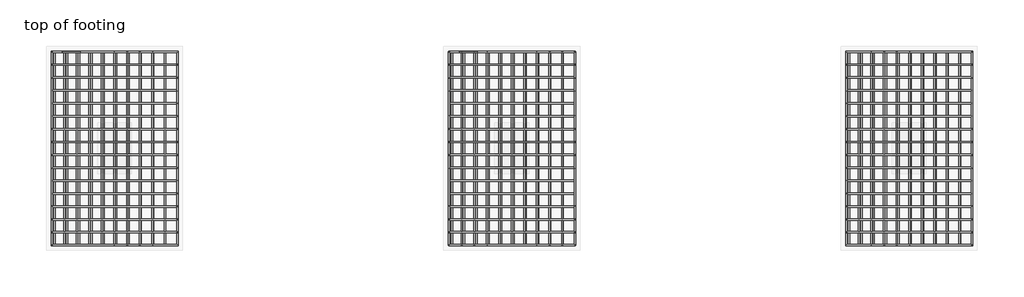
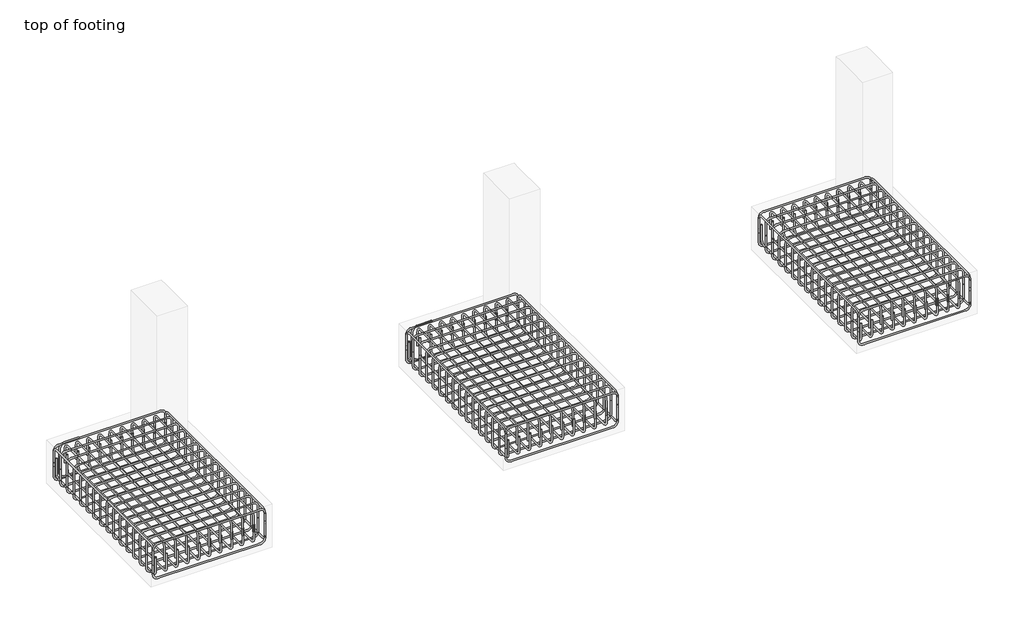
# One storey, part 2 of 8: 14 reinforcing bars.
"""IFC4 building model written with IfcOpenShell, lengths in millimetres."""

from ifc_helpers import new_model, si_unit, point, frame, origin, place, context, project, spatial, polyline, circle_curve, trimmed, segment, composite_curve, source, transform, mapped, element, save
from ifc_brep_helpers import swept_disk

model = new_model("IFC4")

# Units and contexts
model_context = context("Model", 3, world=origin())
ifc_project = project(units=[si_unit("LENGTHUNIT", "METRE", prefix="MILLI")], contexts=[model_context])

# Site, building, storey
site = spatial("IfcSite", under=ifc_project)
building = spatial("IfcBuilding", under=site)
storey = spatial("IfcBuildingStorey", under=building, Name="top of footing", Elevation=-1828.8)

# Reinforcing bars
placement = place(None, origin())
reinforcing_bar_shape = source(origin(), model_context, "Body", "SolidModel", [
    swept_disk(composite_curve([segment(polyline([(-10685.4300189, 4682.8075251, -2014.4920065), (-10685.4300189, 4682.8075251, -2161.7920065)]), True, "CONTINUOUS"), segment(trimmed(circle_curve(frame((-10685.4300189, 4729.1575251, -2161.7920065), z_axis=(1.0, 0.0, 0.0), x_axis=(0.0, -46.350000000000364, 0.0)), 46.35), [point((-10685.4300189, 4682.8075251, -2161.7920065))], [point((-10685.4300189, 4729.1575251, -2208.1420065))], True, "CARTESIAN"), True, "CONTINUOUS"), segment(polyline([(-10685.4300189, 4729.1575251, -2208.1420065), (-10685.4300189, 6343.7575251, -2208.1420065)]), True, "CONTINUOUS"), segment(trimmed(circle_curve(frame((-10685.4300189, 6343.7575251, -2161.7920065), z_axis=(1.0, 0.0, 0.0), x_axis=(0.0, 0.0, -46.350000000000364)), 46.35), [point((-10685.4300189, 6343.7575251, -2208.1420065))], [point((-10685.4300189, 6390.1075251, -2161.7920065))], True, "CARTESIAN"), True, "CONTINUOUS"), segment(polyline([(-10685.4300189, 6390.1075251, -2161.7920065), (-10685.4300189, 6390.1075251, -2014.4920065)]), True, "CONTINUOUS")], self_intersect=False), 6.35),
])
element("IfcReinforcingBar", 1, at=placement, inside=storey, context=model_context, shape_type="MappedRepresentation", body=[
    mapped(reinforcing_bar_shape, transform((0.0, 0.0, 0.0), x_axis=(1.0, 0.0, 0.0), y_axis=(0.0, 1.0, 0.0), z_axis=(0.0, 0.0, 1.0))),
    mapped(reinforcing_bar_shape, transform((-108.3645139, 0.0, 0.0), x_axis=(1.0, 0.0, 0.0), y_axis=(0.0, 1.0, 0.0), z_axis=(0.0, 0.0, 1.0))),
    mapped(reinforcing_bar_shape, transform((-216.7290279, 0.0, 0.0), x_axis=(1.0, 0.0, 0.0), y_axis=(0.0, 1.0, 0.0), z_axis=(0.0, 0.0, 1.0))),
    mapped(reinforcing_bar_shape, transform((-325.0935418, 0.0, 0.0), x_axis=(1.0, 0.0, 0.0), y_axis=(0.0, 1.0, 0.0), z_axis=(0.0, 0.0, 1.0))),
    mapped(reinforcing_bar_shape, transform((-433.4580557, 0.0, 0.0), x_axis=(1.0, 0.0, 0.0), y_axis=(0.0, 1.0, 0.0), z_axis=(0.0, 0.0, 1.0))),
    mapped(reinforcing_bar_shape, transform((-541.8225696, 0.0, 0.0), x_axis=(1.0, 0.0, 0.0), y_axis=(0.0, 1.0, 0.0), z_axis=(0.0, 0.0, 1.0))),
    mapped(reinforcing_bar_shape, transform((-650.1870836, 0.0, 0.0), x_axis=(1.0, 0.0, 0.0), y_axis=(0.0, 1.0, 0.0), z_axis=(0.0, 0.0, 1.0))),
    mapped(reinforcing_bar_shape, transform((-758.5515975, 0.0, 0.0), x_axis=(1.0, 0.0, 0.0), y_axis=(0.0, 1.0, 0.0), z_axis=(0.0, 0.0, 1.0))),
    mapped(reinforcing_bar_shape, transform((-866.9161114, 0.0, 0.0), x_axis=(1.0, 0.0, 0.0), y_axis=(0.0, 1.0, 0.0), z_axis=(0.0, 0.0, 1.0))),
    mapped(reinforcing_bar_shape, transform((-975.2806253, 0.0, 0.0), x_axis=(1.0, 0.0, 0.0), y_axis=(0.0, 1.0, 0.0), z_axis=(0.0, 0.0, 1.0))),
    mapped(reinforcing_bar_shape, transform((-1083.6451393, 0.0, 0.0), x_axis=(1.0, 0.0, 0.0), y_axis=(0.0, 1.0, 0.0), z_axis=(0.0, 0.0, 1.0))),
])
reinforcing_bar_2_shape = source(origin(), model_context, "Body", "SolidModel", [
    swept_disk(composite_curve([segment(polyline([(-11792.7300189, 4682.8075251, -2085.8010212), (-11792.7300189, 4682.8075251, -1938.5010212)]), True, "CONTINUOUS"), segment(trimmed(circle_curve(frame((-11792.7300189, 4729.1575251, -1938.5010212), z_axis=(-1.0, 0.0, 0.0), x_axis=(0.0, -46.350000000000364, 0.0)), 46.35), [point((-11792.7300189, 4682.8075251, -1938.5010212))], [point((-11792.7300189, 4729.1575251, -1892.1510212))], True, "CARTESIAN"), True, "CONTINUOUS"), segment(polyline([(-11792.7300189, 4729.1575251, -1892.1510212), (-11792.7300189, 6343.7575251, -1892.1510212)]), True, "CONTINUOUS"), segment(trimmed(circle_curve(frame((-11792.7300189, 6343.7575251, -1938.5010212), z_axis=(-1.0, 0.0, 0.0), x_axis=(0.0, 0.0, 46.34999999999991)), 46.35), [point((-11792.7300189, 6343.7575251, -1892.1510212))], [point((-11792.7300189, 6390.1075251, -1938.5010212))], True, "CARTESIAN"), True, "CONTINUOUS"), segment(polyline([(-11792.7300189, 6390.1075251, -1938.5010212), (-11792.7300189, 6390.1075251, -2085.8010212)]), True, "CONTINUOUS")], self_intersect=False), 6.35),
])
element("IfcReinforcingBar", 2, at=placement, inside=storey, context=model_context, shape_type="MappedRepresentation", body=[
    mapped(reinforcing_bar_2_shape, transform((0.0, 0.0, 0.0), x_axis=(1.0, 0.0, 0.0), y_axis=(0.0, 1.0, 0.0), z_axis=(0.0, 0.0, 1.0))),
    mapped(reinforcing_bar_2_shape, transform((110.73, 0.0, 0.0), x_axis=(1.0, 0.0, 0.0), y_axis=(0.0, 1.0, 0.0), z_axis=(0.0, 0.0, 1.0))),
    mapped(reinforcing_bar_2_shape, transform((221.46, 0.0, 0.0), x_axis=(1.0, 0.0, 0.0), y_axis=(0.0, 1.0, 0.0), z_axis=(0.0, 0.0, 1.0))),
    mapped(reinforcing_bar_2_shape, transform((332.19, 0.0, 0.0), x_axis=(1.0, 0.0, 0.0), y_axis=(0.0, 1.0, 0.0), z_axis=(0.0, 0.0, 1.0))),
    mapped(reinforcing_bar_2_shape, transform((442.92, 0.0, 0.0), x_axis=(1.0, 0.0, 0.0), y_axis=(0.0, 1.0, 0.0), z_axis=(0.0, 0.0, 1.0))),
    mapped(reinforcing_bar_2_shape, transform((553.65, 0.0, 0.0), x_axis=(1.0, 0.0, 0.0), y_axis=(0.0, 1.0, 0.0), z_axis=(0.0, 0.0, 1.0))),
    mapped(reinforcing_bar_2_shape, transform((664.38, 0.0, 0.0), x_axis=(1.0, 0.0, 0.0), y_axis=(0.0, 1.0, 0.0), z_axis=(0.0, 0.0, 1.0))),
    mapped(reinforcing_bar_2_shape, transform((775.11, 0.0, 0.0), x_axis=(1.0, 0.0, 0.0), y_axis=(0.0, 1.0, 0.0), z_axis=(0.0, 0.0, 1.0))),
    mapped(reinforcing_bar_2_shape, transform((885.84, 0.0, 0.0), x_axis=(1.0, 0.0, 0.0), y_axis=(0.0, 1.0, 0.0), z_axis=(0.0, 0.0, 1.0))),
    mapped(reinforcing_bar_2_shape, transform((996.57, 0.0, 0.0), x_axis=(1.0, 0.0, 0.0), y_axis=(0.0, 1.0, 0.0), z_axis=(0.0, 0.0, 1.0))),
    mapped(reinforcing_bar_2_shape, transform((1107.3, 0.0, 0.0), x_axis=(1.0, 0.0, 0.0), y_axis=(0.0, 1.0, 0.0), z_axis=(0.0, 0.0, 1.0))),
])
element("IfcReinforcingBar", 3, at=placement, inside=storey, context=model_context, shape_type="SolidModel", body=[
    swept_disk(composite_curve([segment(polyline([(-11543.0309105, 6390.1075251, -2232.45), (-11690.3309105, 6390.1075251, -2232.45)]), True, "CONTINUOUS"), segment(trimmed(circle_curve(frame((-11690.3309105, 6390.1075251, -2186.1), z_axis=(0.0, 1.0, 0.0), x_axis=(0.0, 0.0, -46.34999999999991)), 46.35), [point((-11690.3309105, 6390.1075251, -2232.45))], [point((-11736.6809105, 6390.1075251, -2186.1))], True, "CARTESIAN"), True, "CONTINUOUS"), segment(polyline([(-11736.6809105, 6390.1075251, -2186.1), (-11736.6809105, 6390.1075251, -1921.5)]), True, "CONTINUOUS"), segment(trimmed(circle_curve(frame((-11690.3309105, 6390.1075251, -1921.5), z_axis=(0.0, 1.0, 0.0), x_axis=(-46.349999999998545, 0.0, 0.0)), 46.35), [point((-11736.6809105, 6390.1075251, -1921.5))], [point((-11690.3309105, 6390.1075251, -1875.15))], True, "CARTESIAN"), True, "CONTINUOUS"), segment(polyline([(-11690.3309105, 6390.1075251, -1875.15), (-11543.0309105, 6390.1075251, -1875.15)]), True, "CONTINUOUS")], self_intersect=False), 6.35),
])
reinforcing_bar_3_shape = source(origin(), model_context, "Body", "SolidModel", [
    swept_disk(composite_curve([segment(polyline([(-10685.4300189, 6390.1075251, -2044.8290141), (-10685.4300189, 6390.1075251, -2192.1290141)]), True, "CONTINUOUS"), segment(trimmed(circle_curve(frame((-10731.7800189, 6390.1075251, -2192.1290141), z_axis=(0.0, 1.0, 0.0), x_axis=(46.350000000000364, 0.0, 0.0)), 46.35), [point((-10685.4300189, 6390.1075251, -2192.1290141))], [point((-10731.7800189, 6390.1075251, -2238.4790141))], True, "CARTESIAN"), True, "CONTINUOUS"), segment(polyline([(-10731.7800189, 6390.1075251, -2238.4790141), (-11746.3800189, 6390.1075251, -2238.4790141)]), True, "CONTINUOUS"), segment(trimmed(circle_curve(frame((-11746.3800189, 6390.1075251, -2192.1290141), z_axis=(0.0, 1.0, 0.0), x_axis=(0.0, 0.0, -46.34999999999991)), 46.35), [point((-11746.3800189, 6390.1075251, -2238.4790141))], [point((-11792.7300189, 6390.1075251, -2192.1290141))], True, "CARTESIAN"), True, "CONTINUOUS"), segment(polyline([(-11792.7300189, 6390.1075251, -2192.1290141), (-11792.7300189, 6390.1075251, -2044.8290141)]), True, "CONTINUOUS")], self_intersect=False), 6.35),
])
element("IfcReinforcingBar", 4, at=placement, inside=storey, context=model_context, shape_type="MappedRepresentation", body=[
    mapped(reinforcing_bar_3_shape, transform((0.0, 0.0, 0.0), x_axis=(1.0, 0.0, 0.0), y_axis=(0.0, 1.0, 0.0), z_axis=(0.0, 0.0, 1.0))),
    mapped(reinforcing_bar_3_shape, transform((0.0, -113.82, 0.0), x_axis=(1.0, 0.0, 0.0), y_axis=(0.0, 1.0, 0.0), z_axis=(0.0, 0.0, 1.0))),
    mapped(reinforcing_bar_3_shape, transform((0.0, -227.64, 0.0), x_axis=(1.0, 0.0, 0.0), y_axis=(0.0, 1.0, 0.0), z_axis=(0.0, 0.0, 1.0))),
    mapped(reinforcing_bar_3_shape, transform((0.0, -341.46, 0.0), x_axis=(1.0, 0.0, 0.0), y_axis=(0.0, 1.0, 0.0), z_axis=(0.0, 0.0, 1.0))),
    mapped(reinforcing_bar_3_shape, transform((0.0, -455.28, 0.0), x_axis=(1.0, 0.0, 0.0), y_axis=(0.0, 1.0, 0.0), z_axis=(0.0, 0.0, 1.0))),
    mapped(reinforcing_bar_3_shape, transform((0.0, -569.1, 0.0), x_axis=(1.0, 0.0, 0.0), y_axis=(0.0, 1.0, 0.0), z_axis=(0.0, 0.0, 1.0))),
    mapped(reinforcing_bar_3_shape, transform((0.0, -682.92, 0.0), x_axis=(1.0, 0.0, 0.0), y_axis=(0.0, 1.0, 0.0), z_axis=(0.0, 0.0, 1.0))),
    mapped(reinforcing_bar_3_shape, transform((0.0, -796.74, 0.0), x_axis=(1.0, 0.0, 0.0), y_axis=(0.0, 1.0, 0.0), z_axis=(0.0, 0.0, 1.0))),
    mapped(reinforcing_bar_3_shape, transform((0.0, -910.56, 0.0), x_axis=(1.0, 0.0, 0.0), y_axis=(0.0, 1.0, 0.0), z_axis=(0.0, 0.0, 1.0))),
    mapped(reinforcing_bar_3_shape, transform((0.0, -1024.38, 0.0), x_axis=(1.0, 0.0, 0.0), y_axis=(0.0, 1.0, 0.0), z_axis=(0.0, 0.0, 1.0))),
    mapped(reinforcing_bar_3_shape, transform((0.0, -1138.2, 0.0), x_axis=(1.0, 0.0, 0.0), y_axis=(0.0, 1.0, 0.0), z_axis=(0.0, 0.0, 1.0))),
    mapped(reinforcing_bar_3_shape, transform((0.0, -1252.02, 0.0), x_axis=(1.0, 0.0, 0.0), y_axis=(0.0, 1.0, 0.0), z_axis=(0.0, 0.0, 1.0))),
    mapped(reinforcing_bar_3_shape, transform((0.0, -1365.84, 0.0), x_axis=(1.0, 0.0, 0.0), y_axis=(0.0, 1.0, 0.0), z_axis=(0.0, 0.0, 1.0))),
    mapped(reinforcing_bar_3_shape, transform((0.0, -1479.66, 0.0), x_axis=(1.0, 0.0, 0.0), y_axis=(0.0, 1.0, 0.0), z_axis=(0.0, 0.0, 1.0))),
    mapped(reinforcing_bar_3_shape, transform((0.0, -1593.48, 0.0), x_axis=(1.0, 0.0, 0.0), y_axis=(0.0, 1.0, 0.0), z_axis=(0.0, 0.0, 1.0))),
    mapped(reinforcing_bar_3_shape, transform((0.0, -1707.3, 0.0), x_axis=(1.0, 0.0, 0.0), y_axis=(0.0, 1.0, 0.0), z_axis=(0.0, 0.0, 1.0))),
])
reinforcing_bar_4_shape = source(origin(), model_context, "Body", "SolidModel", [
    swept_disk(composite_curve([segment(polyline([(-11792.7300189, 6390.1075251, -2075.0801535), (-11792.7300189, 6390.1075251, -1927.7801535)]), True, "CONTINUOUS"), segment(trimmed(circle_curve(frame((-11746.3800189, 6390.1075251, -1927.7801535), z_axis=(0.0, 1.0, 0.0), x_axis=(-46.350000000000364, 0.0, 0.0)), 46.35), [point((-11792.7300189, 6390.1075251, -1927.7801535))], [point((-11746.3800189, 6390.1075251, -1881.4301535))], True, "CARTESIAN"), True, "CONTINUOUS"), segment(polyline([(-11746.3800189, 6390.1075251, -1881.4301535), (-10731.7800189, 6390.1075251, -1881.4301535)]), True, "CONTINUOUS"), segment(trimmed(circle_curve(frame((-10731.7800189, 6390.1075251, -1927.7801535), z_axis=(0.0, 1.0, 0.0), x_axis=(0.0, 0.0, 46.350000000000136)), 46.35), [point((-10731.7800189, 6390.1075251, -1881.4301535))], [point((-10685.4300189, 6390.1075251, -1927.7801535))], True, "CARTESIAN"), True, "CONTINUOUS"), segment(polyline([(-10685.4300189, 6390.1075251, -1927.7801535), (-10685.4300189, 6390.1075251, -2075.0801535)]), True, "CONTINUOUS")], self_intersect=False), 6.35),
])
element("IfcReinforcingBar", 5, at=placement, inside=storey, context=model_context, shape_type="MappedRepresentation", body=[
    mapped(reinforcing_bar_4_shape, transform((0.0, 0.0, 0.0), x_axis=(1.0, 0.0, 0.0), y_axis=(0.0, 1.0, 0.0), z_axis=(0.0, 0.0, 1.0))),
    mapped(reinforcing_bar_4_shape, transform((0.0, -113.82, 0.0), x_axis=(1.0, 0.0, 0.0), y_axis=(0.0, 1.0, 0.0), z_axis=(0.0, 0.0, 1.0))),
    mapped(reinforcing_bar_4_shape, transform((0.0, -227.64, 0.0), x_axis=(1.0, 0.0, 0.0), y_axis=(0.0, 1.0, 0.0), z_axis=(0.0, 0.0, 1.0))),
    mapped(reinforcing_bar_4_shape, transform((0.0, -341.46, 0.0), x_axis=(1.0, 0.0, 0.0), y_axis=(0.0, 1.0, 0.0), z_axis=(0.0, 0.0, 1.0))),
    mapped(reinforcing_bar_4_shape, transform((0.0, -455.28, 0.0), x_axis=(1.0, 0.0, 0.0), y_axis=(0.0, 1.0, 0.0), z_axis=(0.0, 0.0, 1.0))),
    mapped(reinforcing_bar_4_shape, transform((0.0, -569.1, 0.0), x_axis=(1.0, 0.0, 0.0), y_axis=(0.0, 1.0, 0.0), z_axis=(0.0, 0.0, 1.0))),
    mapped(reinforcing_bar_4_shape, transform((0.0, -682.92, 0.0), x_axis=(1.0, 0.0, 0.0), y_axis=(0.0, 1.0, 0.0), z_axis=(0.0, 0.0, 1.0))),
    mapped(reinforcing_bar_4_shape, transform((0.0, -796.74, 0.0), x_axis=(1.0, 0.0, 0.0), y_axis=(0.0, 1.0, 0.0), z_axis=(0.0, 0.0, 1.0))),
    mapped(reinforcing_bar_4_shape, transform((0.0, -910.56, 0.0), x_axis=(1.0, 0.0, 0.0), y_axis=(0.0, 1.0, 0.0), z_axis=(0.0, 0.0, 1.0))),
    mapped(reinforcing_bar_4_shape, transform((0.0, -1024.38, 0.0), x_axis=(1.0, 0.0, 0.0), y_axis=(0.0, 1.0, 0.0), z_axis=(0.0, 0.0, 1.0))),
    mapped(reinforcing_bar_4_shape, transform((0.0, -1138.2, 0.0), x_axis=(1.0, 0.0, 0.0), y_axis=(0.0, 1.0, 0.0), z_axis=(0.0, 0.0, 1.0))),
    mapped(reinforcing_bar_4_shape, transform((0.0, -1252.02, 0.0), x_axis=(1.0, 0.0, 0.0), y_axis=(0.0, 1.0, 0.0), z_axis=(0.0, 0.0, 1.0))),
    mapped(reinforcing_bar_4_shape, transform((0.0, -1365.84, 0.0), x_axis=(1.0, 0.0, 0.0), y_axis=(0.0, 1.0, 0.0), z_axis=(0.0, 0.0, 1.0))),
    mapped(reinforcing_bar_4_shape, transform((0.0, -1479.66, 0.0), x_axis=(1.0, 0.0, 0.0), y_axis=(0.0, 1.0, 0.0), z_axis=(0.0, 0.0, 1.0))),
    mapped(reinforcing_bar_4_shape, transform((0.0, -1593.48, 0.0), x_axis=(1.0, 0.0, 0.0), y_axis=(0.0, 1.0, 0.0), z_axis=(0.0, 0.0, 1.0))),
    mapped(reinforcing_bar_4_shape, transform((0.0, -1707.3, 0.0), x_axis=(1.0, 0.0, 0.0), y_axis=(0.0, 1.0, 0.0), z_axis=(0.0, 0.0, 1.0))),
])
reinforcing_bar_5_shape = source(origin(), model_context, "Body", "SolidModel", [
    swept_disk(composite_curve([segment(polyline([(-7185.4300189, 4682.8075251, -2014.4920065), (-7185.4300189, 4682.8075251, -2161.7920065)]), True, "CONTINUOUS"), segment(trimmed(circle_curve(frame((-7185.4300189, 4729.1575251, -2161.7920065), z_axis=(1.0, 0.0, 0.0), x_axis=(0.0, -46.350000000000364, 0.0)), 46.35), [point((-7185.4300189, 4682.8075251, -2161.7920065))], [point((-7185.4300189, 4729.1575251, -2208.1420065))], True, "CARTESIAN"), True, "CONTINUOUS"), segment(polyline([(-7185.4300189, 4729.1575251, -2208.1420065), (-7185.4300189, 6343.7575251, -2208.1420065)]), True, "CONTINUOUS"), segment(trimmed(circle_curve(frame((-7185.4300189, 6343.7575251, -2161.7920065), z_axis=(1.0, 0.0, 0.0), x_axis=(0.0, 0.0, -46.350000000000364)), 46.35), [point((-7185.4300189, 6343.7575251, -2208.1420065))], [point((-7185.4300189, 6390.1075251, -2161.7920065))], True, "CARTESIAN"), True, "CONTINUOUS"), segment(polyline([(-7185.4300189, 6390.1075251, -2161.7920065), (-7185.4300189, 6390.1075251, -2014.4920065)]), True, "CONTINUOUS")], self_intersect=False), 6.35),
])
element("IfcReinforcingBar", 6, at=placement, inside=storey, context=model_context, shape_type="MappedRepresentation", body=[
    mapped(reinforcing_bar_5_shape, transform((0.0, 0.0, 0.0), x_axis=(1.0, 0.0, 0.0), y_axis=(0.0, 1.0, 0.0), z_axis=(0.0, 0.0, 1.0))),
    mapped(reinforcing_bar_5_shape, transform((-108.3645139, 0.0, 0.0), x_axis=(1.0, 0.0, 0.0), y_axis=(0.0, 1.0, 0.0), z_axis=(0.0, 0.0, 1.0))),
    mapped(reinforcing_bar_5_shape, transform((-216.7290279, 0.0, 0.0), x_axis=(1.0, 0.0, 0.0), y_axis=(0.0, 1.0, 0.0), z_axis=(0.0, 0.0, 1.0))),
    mapped(reinforcing_bar_5_shape, transform((-325.0935418, 0.0, 0.0), x_axis=(1.0, 0.0, 0.0), y_axis=(0.0, 1.0, 0.0), z_axis=(0.0, 0.0, 1.0))),
    mapped(reinforcing_bar_5_shape, transform((-433.4580557, 0.0, 0.0), x_axis=(1.0, 0.0, 0.0), y_axis=(0.0, 1.0, 0.0), z_axis=(0.0, 0.0, 1.0))),
    mapped(reinforcing_bar_5_shape, transform((-541.8225696, 0.0, 0.0), x_axis=(1.0, 0.0, 0.0), y_axis=(0.0, 1.0, 0.0), z_axis=(0.0, 0.0, 1.0))),
    mapped(reinforcing_bar_5_shape, transform((-650.1870836, 0.0, 0.0), x_axis=(1.0, 0.0, 0.0), y_axis=(0.0, 1.0, 0.0), z_axis=(0.0, 0.0, 1.0))),
    mapped(reinforcing_bar_5_shape, transform((-758.5515975, 0.0, 0.0), x_axis=(1.0, 0.0, 0.0), y_axis=(0.0, 1.0, 0.0), z_axis=(0.0, 0.0, 1.0))),
    mapped(reinforcing_bar_5_shape, transform((-866.9161114, 0.0, 0.0), x_axis=(1.0, 0.0, 0.0), y_axis=(0.0, 1.0, 0.0), z_axis=(0.0, 0.0, 1.0))),
    mapped(reinforcing_bar_5_shape, transform((-975.2806253, 0.0, 0.0), x_axis=(1.0, 0.0, 0.0), y_axis=(0.0, 1.0, 0.0), z_axis=(0.0, 0.0, 1.0))),
    mapped(reinforcing_bar_5_shape, transform((-1083.6451393, 0.0, 0.0), x_axis=(1.0, 0.0, 0.0), y_axis=(0.0, 1.0, 0.0), z_axis=(0.0, 0.0, 1.0))),
])
reinforcing_bar_6_shape = source(origin(), model_context, "Body", "SolidModel", [
    swept_disk(composite_curve([segment(polyline([(-8292.7300189, 4682.8075251, -2085.8010212), (-8292.7300189, 4682.8075251, -1938.5010212)]), True, "CONTINUOUS"), segment(trimmed(circle_curve(frame((-8292.7300189, 4729.1575251, -1938.5010212), z_axis=(-1.0, 0.0, 0.0), x_axis=(0.0, -46.350000000000364, 0.0)), 46.35), [point((-8292.7300189, 4682.8075251, -1938.5010212))], [point((-8292.7300189, 4729.1575251, -1892.1510212))], True, "CARTESIAN"), True, "CONTINUOUS"), segment(polyline([(-8292.7300189, 4729.1575251, -1892.1510212), (-8292.7300189, 6343.7575251, -1892.1510212)]), True, "CONTINUOUS"), segment(trimmed(circle_curve(frame((-8292.7300189, 6343.7575251, -1938.5010212), z_axis=(-1.0, 0.0, 0.0), x_axis=(0.0, 0.0, 46.34999999999991)), 46.35), [point((-8292.7300189, 6343.7575251, -1892.1510212))], [point((-8292.7300189, 6390.1075251, -1938.5010212))], True, "CARTESIAN"), True, "CONTINUOUS"), segment(polyline([(-8292.7300189, 6390.1075251, -1938.5010212), (-8292.7300189, 6390.1075251, -2085.8010212)]), True, "CONTINUOUS")], self_intersect=False), 6.35),
])
element("IfcReinforcingBar", 7, at=placement, inside=storey, context=model_context, shape_type="MappedRepresentation", body=[
    mapped(reinforcing_bar_6_shape, transform((0.0, 0.0, 0.0), x_axis=(1.0, 0.0, 0.0), y_axis=(0.0, 1.0, 0.0), z_axis=(0.0, 0.0, 1.0))),
    mapped(reinforcing_bar_6_shape, transform((110.73, 0.0, 0.0), x_axis=(1.0, 0.0, 0.0), y_axis=(0.0, 1.0, 0.0), z_axis=(0.0, 0.0, 1.0))),
    mapped(reinforcing_bar_6_shape, transform((221.46, 0.0, 0.0), x_axis=(1.0, 0.0, 0.0), y_axis=(0.0, 1.0, 0.0), z_axis=(0.0, 0.0, 1.0))),
    mapped(reinforcing_bar_6_shape, transform((332.19, 0.0, 0.0), x_axis=(1.0, 0.0, 0.0), y_axis=(0.0, 1.0, 0.0), z_axis=(0.0, 0.0, 1.0))),
    mapped(reinforcing_bar_6_shape, transform((442.92, 0.0, 0.0), x_axis=(1.0, 0.0, 0.0), y_axis=(0.0, 1.0, 0.0), z_axis=(0.0, 0.0, 1.0))),
    mapped(reinforcing_bar_6_shape, transform((553.65, 0.0, 0.0), x_axis=(1.0, 0.0, 0.0), y_axis=(0.0, 1.0, 0.0), z_axis=(0.0, 0.0, 1.0))),
    mapped(reinforcing_bar_6_shape, transform((664.38, 0.0, 0.0), x_axis=(1.0, 0.0, 0.0), y_axis=(0.0, 1.0, 0.0), z_axis=(0.0, 0.0, 1.0))),
    mapped(reinforcing_bar_6_shape, transform((775.11, 0.0, 0.0), x_axis=(1.0, 0.0, 0.0), y_axis=(0.0, 1.0, 0.0), z_axis=(0.0, 0.0, 1.0))),
    mapped(reinforcing_bar_6_shape, transform((885.84, 0.0, 0.0), x_axis=(1.0, 0.0, 0.0), y_axis=(0.0, 1.0, 0.0), z_axis=(0.0, 0.0, 1.0))),
    mapped(reinforcing_bar_6_shape, transform((996.57, 0.0, 0.0), x_axis=(1.0, 0.0, 0.0), y_axis=(0.0, 1.0, 0.0), z_axis=(0.0, 0.0, 1.0))),
    mapped(reinforcing_bar_6_shape, transform((1107.3, 0.0, 0.0), x_axis=(1.0, 0.0, 0.0), y_axis=(0.0, 1.0, 0.0), z_axis=(0.0, 0.0, 1.0))),
])
element("IfcReinforcingBar", 8, at=placement, inside=storey, context=model_context, shape_type="SolidModel", body=[
    swept_disk(composite_curve([segment(polyline([(-8043.0309105, 6390.1075251, -2232.45), (-8190.3309105, 6390.1075251, -2232.45)]), True, "CONTINUOUS"), segment(trimmed(circle_curve(frame((-8190.3309105, 6390.1075251, -2186.1), z_axis=(0.0, 1.0, 0.0), x_axis=(0.0, 0.0, -46.34999999999991)), 46.35), [point((-8190.3309105, 6390.1075251, -2232.45))], [point((-8236.6809105, 6390.1075251, -2186.1))], True, "CARTESIAN"), True, "CONTINUOUS"), segment(polyline([(-8236.6809105, 6390.1075251, -2186.1), (-8236.6809105, 6390.1075251, -1921.5)]), True, "CONTINUOUS"), segment(trimmed(circle_curve(frame((-8190.3309105, 6390.1075251, -1921.5), z_axis=(0.0, 1.0, 0.0), x_axis=(-46.349999999999454, 0.0, 0.0)), 46.35), [point((-8236.6809105, 6390.1075251, -1921.5))], [point((-8190.3309105, 6390.1075251, -1875.15))], True, "CARTESIAN"), True, "CONTINUOUS"), segment(polyline([(-8190.3309105, 6390.1075251, -1875.15), (-8043.0309105, 6390.1075251, -1875.15)]), True, "CONTINUOUS")], self_intersect=False), 6.35),
])
reinforcing_bar_7_shape = source(origin(), model_context, "Body", "SolidModel", [
    swept_disk(composite_curve([segment(polyline([(-7185.4300189, 6390.1075251, -2044.8290141), (-7185.4300189, 6390.1075251, -2192.1290141)]), True, "CONTINUOUS"), segment(trimmed(circle_curve(frame((-7231.7800189, 6390.1075251, -2192.1290141), z_axis=(0.0, 1.0, 0.0), x_axis=(46.350000000000364, 0.0, 0.0)), 46.35), [point((-7185.4300189, 6390.1075251, -2192.1290141))], [point((-7231.7800189, 6390.1075251, -2238.4790141))], True, "CARTESIAN"), True, "CONTINUOUS"), segment(polyline([(-7231.7800189, 6390.1075251, -2238.4790141), (-8246.3800189, 6390.1075251, -2238.4790141)]), True, "CONTINUOUS"), segment(trimmed(circle_curve(frame((-8246.3800189, 6390.1075251, -2192.1290141), z_axis=(0.0, 1.0, 0.0), x_axis=(0.0, 0.0, -46.34999999999991)), 46.35), [point((-8246.3800189, 6390.1075251, -2238.4790141))], [point((-8292.7300189, 6390.1075251, -2192.1290141))], True, "CARTESIAN"), True, "CONTINUOUS"), segment(polyline([(-8292.7300189, 6390.1075251, -2192.1290141), (-8292.7300189, 6390.1075251, -2044.8290141)]), True, "CONTINUOUS")], self_intersect=False), 6.35),
])
element("IfcReinforcingBar", 9, at=placement, inside=storey, context=model_context, shape_type="MappedRepresentation", body=[
    mapped(reinforcing_bar_7_shape, transform((0.0, 0.0, 0.0), x_axis=(1.0, 0.0, 0.0), y_axis=(0.0, 1.0, 0.0), z_axis=(0.0, 0.0, 1.0))),
    mapped(reinforcing_bar_7_shape, transform((0.0, -113.82, 0.0), x_axis=(1.0, 0.0, 0.0), y_axis=(0.0, 1.0, 0.0), z_axis=(0.0, 0.0, 1.0))),
    mapped(reinforcing_bar_7_shape, transform((0.0, -227.64, 0.0), x_axis=(1.0, 0.0, 0.0), y_axis=(0.0, 1.0, 0.0), z_axis=(0.0, 0.0, 1.0))),
    mapped(reinforcing_bar_7_shape, transform((0.0, -341.46, 0.0), x_axis=(1.0, 0.0, 0.0), y_axis=(0.0, 1.0, 0.0), z_axis=(0.0, 0.0, 1.0))),
    mapped(reinforcing_bar_7_shape, transform((0.0, -455.28, 0.0), x_axis=(1.0, 0.0, 0.0), y_axis=(0.0, 1.0, 0.0), z_axis=(0.0, 0.0, 1.0))),
    mapped(reinforcing_bar_7_shape, transform((0.0, -569.1, 0.0), x_axis=(1.0, 0.0, 0.0), y_axis=(0.0, 1.0, 0.0), z_axis=(0.0, 0.0, 1.0))),
    mapped(reinforcing_bar_7_shape, transform((0.0, -682.92, 0.0), x_axis=(1.0, 0.0, 0.0), y_axis=(0.0, 1.0, 0.0), z_axis=(0.0, 0.0, 1.0))),
    mapped(reinforcing_bar_7_shape, transform((0.0, -796.74, 0.0), x_axis=(1.0, 0.0, 0.0), y_axis=(0.0, 1.0, 0.0), z_axis=(0.0, 0.0, 1.0))),
    mapped(reinforcing_bar_7_shape, transform((0.0, -910.56, 0.0), x_axis=(1.0, 0.0, 0.0), y_axis=(0.0, 1.0, 0.0), z_axis=(0.0, 0.0, 1.0))),
    mapped(reinforcing_bar_7_shape, transform((0.0, -1024.38, 0.0), x_axis=(1.0, 0.0, 0.0), y_axis=(0.0, 1.0, 0.0), z_axis=(0.0, 0.0, 1.0))),
    mapped(reinforcing_bar_7_shape, transform((0.0, -1138.2, 0.0), x_axis=(1.0, 0.0, 0.0), y_axis=(0.0, 1.0, 0.0), z_axis=(0.0, 0.0, 1.0))),
    mapped(reinforcing_bar_7_shape, transform((0.0, -1252.02, 0.0), x_axis=(1.0, 0.0, 0.0), y_axis=(0.0, 1.0, 0.0), z_axis=(0.0, 0.0, 1.0))),
    mapped(reinforcing_bar_7_shape, transform((0.0, -1365.84, 0.0), x_axis=(1.0, 0.0, 0.0), y_axis=(0.0, 1.0, 0.0), z_axis=(0.0, 0.0, 1.0))),
    mapped(reinforcing_bar_7_shape, transform((0.0, -1479.66, 0.0), x_axis=(1.0, 0.0, 0.0), y_axis=(0.0, 1.0, 0.0), z_axis=(0.0, 0.0, 1.0))),
    mapped(reinforcing_bar_7_shape, transform((0.0, -1593.48, 0.0), x_axis=(1.0, 0.0, 0.0), y_axis=(0.0, 1.0, 0.0), z_axis=(0.0, 0.0, 1.0))),
    mapped(reinforcing_bar_7_shape, transform((0.0, -1707.3, 0.0), x_axis=(1.0, 0.0, 0.0), y_axis=(0.0, 1.0, 0.0), z_axis=(0.0, 0.0, 1.0))),
])
reinforcing_bar_8_shape = source(origin(), model_context, "Body", "SolidModel", [
    swept_disk(composite_curve([segment(polyline([(-8292.7300189, 6390.1075251, -2075.0801535), (-8292.7300189, 6390.1075251, -1927.7801535)]), True, "CONTINUOUS"), segment(trimmed(circle_curve(frame((-8246.3800189, 6390.1075251, -1927.7801535), z_axis=(0.0, 1.0, 0.0), x_axis=(-46.350000000000364, 0.0, 0.0)), 46.35), [point((-8292.7300189, 6390.1075251, -1927.7801535))], [point((-8246.3800189, 6390.1075251, -1881.4301535))], True, "CARTESIAN"), True, "CONTINUOUS"), segment(polyline([(-8246.3800189, 6390.1075251, -1881.4301535), (-7231.7800189, 6390.1075251, -1881.4301535)]), True, "CONTINUOUS"), segment(trimmed(circle_curve(frame((-7231.7800189, 6390.1075251, -1927.7801535), z_axis=(0.0, 1.0, 0.0), x_axis=(0.0, 0.0, 46.350000000000136)), 46.35), [point((-7231.7800189, 6390.1075251, -1881.4301535))], [point((-7185.4300189, 6390.1075251, -1927.7801535))], True, "CARTESIAN"), True, "CONTINUOUS"), segment(polyline([(-7185.4300189, 6390.1075251, -1927.7801535), (-7185.4300189, 6390.1075251, -2075.0801535)]), True, "CONTINUOUS")], self_intersect=False), 6.35),
])
element("IfcReinforcingBar", 10, at=placement, inside=storey, context=model_context, shape_type="MappedRepresentation", body=[
    mapped(reinforcing_bar_8_shape, transform((0.0, 0.0, 0.0), x_axis=(1.0, 0.0, 0.0), y_axis=(0.0, 1.0, 0.0), z_axis=(0.0, 0.0, 1.0))),
    mapped(reinforcing_bar_8_shape, transform((0.0, -113.82, 0.0), x_axis=(1.0, 0.0, 0.0), y_axis=(0.0, 1.0, 0.0), z_axis=(0.0, 0.0, 1.0))),
    mapped(reinforcing_bar_8_shape, transform((0.0, -227.64, 0.0), x_axis=(1.0, 0.0, 0.0), y_axis=(0.0, 1.0, 0.0), z_axis=(0.0, 0.0, 1.0))),
    mapped(reinforcing_bar_8_shape, transform((0.0, -341.46, 0.0), x_axis=(1.0, 0.0, 0.0), y_axis=(0.0, 1.0, 0.0), z_axis=(0.0, 0.0, 1.0))),
    mapped(reinforcing_bar_8_shape, transform((0.0, -455.28, 0.0), x_axis=(1.0, 0.0, 0.0), y_axis=(0.0, 1.0, 0.0), z_axis=(0.0, 0.0, 1.0))),
    mapped(reinforcing_bar_8_shape, transform((0.0, -569.1, 0.0), x_axis=(1.0, 0.0, 0.0), y_axis=(0.0, 1.0, 0.0), z_axis=(0.0, 0.0, 1.0))),
    mapped(reinforcing_bar_8_shape, transform((0.0, -682.92, 0.0), x_axis=(1.0, 0.0, 0.0), y_axis=(0.0, 1.0, 0.0), z_axis=(0.0, 0.0, 1.0))),
    mapped(reinforcing_bar_8_shape, transform((0.0, -796.74, 0.0), x_axis=(1.0, 0.0, 0.0), y_axis=(0.0, 1.0, 0.0), z_axis=(0.0, 0.0, 1.0))),
    mapped(reinforcing_bar_8_shape, transform((0.0, -910.56, 0.0), x_axis=(1.0, 0.0, 0.0), y_axis=(0.0, 1.0, 0.0), z_axis=(0.0, 0.0, 1.0))),
    mapped(reinforcing_bar_8_shape, transform((0.0, -1024.38, 0.0), x_axis=(1.0, 0.0, 0.0), y_axis=(0.0, 1.0, 0.0), z_axis=(0.0, 0.0, 1.0))),
    mapped(reinforcing_bar_8_shape, transform((0.0, -1138.2, 0.0), x_axis=(1.0, 0.0, 0.0), y_axis=(0.0, 1.0, 0.0), z_axis=(0.0, 0.0, 1.0))),
    mapped(reinforcing_bar_8_shape, transform((0.0, -1252.02, 0.0), x_axis=(1.0, 0.0, 0.0), y_axis=(0.0, 1.0, 0.0), z_axis=(0.0, 0.0, 1.0))),
    mapped(reinforcing_bar_8_shape, transform((0.0, -1365.84, 0.0), x_axis=(1.0, 0.0, 0.0), y_axis=(0.0, 1.0, 0.0), z_axis=(0.0, 0.0, 1.0))),
    mapped(reinforcing_bar_8_shape, transform((0.0, -1479.66, 0.0), x_axis=(1.0, 0.0, 0.0), y_axis=(0.0, 1.0, 0.0), z_axis=(0.0, 0.0, 1.0))),
    mapped(reinforcing_bar_8_shape, transform((0.0, -1593.48, 0.0), x_axis=(1.0, 0.0, 0.0), y_axis=(0.0, 1.0, 0.0), z_axis=(0.0, 0.0, 1.0))),
    mapped(reinforcing_bar_8_shape, transform((0.0, -1707.3, 0.0), x_axis=(1.0, 0.0, 0.0), y_axis=(0.0, 1.0, 0.0), z_axis=(0.0, 0.0, 1.0))),
])
reinforcing_bar_9_shape = source(origin(), model_context, "Body", "SolidModel", [
    swept_disk(composite_curve([segment(polyline([(-3685.4300189, 4682.8075251, -2014.4920065), (-3685.4300189, 4682.8075251, -2161.7920065)]), True, "CONTINUOUS"), segment(trimmed(circle_curve(frame((-3685.4300189, 4729.1575251, -2161.7920065), z_axis=(1.0, 0.0, 0.0), x_axis=(0.0, -46.350000000000364, 0.0)), 46.35), [point((-3685.4300189, 4682.8075251, -2161.7920065))], [point((-3685.4300189, 4729.1575251, -2208.1420065))], True, "CARTESIAN"), True, "CONTINUOUS"), segment(polyline([(-3685.4300189, 4729.1575251, -2208.1420065), (-3685.4300189, 6343.7575251, -2208.1420065)]), True, "CONTINUOUS"), segment(trimmed(circle_curve(frame((-3685.4300189, 6343.7575251, -2161.7920065), z_axis=(1.0, 0.0, 0.0), x_axis=(0.0, 0.0, -46.350000000000364)), 46.35), [point((-3685.4300189, 6343.7575251, -2208.1420065))], [point((-3685.4300189, 6390.1075251, -2161.7920065))], True, "CARTESIAN"), True, "CONTINUOUS"), segment(polyline([(-3685.4300189, 6390.1075251, -2161.7920065), (-3685.4300189, 6390.1075251, -2014.4920065)]), True, "CONTINUOUS")], self_intersect=False), 6.35),
])
element("IfcReinforcingBar", 11, at=placement, inside=storey, context=model_context, shape_type="MappedRepresentation", body=[
    mapped(reinforcing_bar_9_shape, transform((0.0, 0.0, 0.0), x_axis=(1.0, 0.0, 0.0), y_axis=(0.0, 1.0, 0.0), z_axis=(0.0, 0.0, 1.0))),
    mapped(reinforcing_bar_9_shape, transform((-108.3645139, 0.0, 0.0), x_axis=(1.0, 0.0, 0.0), y_axis=(0.0, 1.0, 0.0), z_axis=(0.0, 0.0, 1.0))),
    mapped(reinforcing_bar_9_shape, transform((-216.7290279, 0.0, 0.0), x_axis=(1.0, 0.0, 0.0), y_axis=(0.0, 1.0, 0.0), z_axis=(0.0, 0.0, 1.0))),
    mapped(reinforcing_bar_9_shape, transform((-325.0935418, 0.0, 0.0), x_axis=(1.0, 0.0, 0.0), y_axis=(0.0, 1.0, 0.0), z_axis=(0.0, 0.0, 1.0))),
    mapped(reinforcing_bar_9_shape, transform((-433.4580557, 0.0, 0.0), x_axis=(1.0, 0.0, 0.0), y_axis=(0.0, 1.0, 0.0), z_axis=(0.0, 0.0, 1.0))),
    mapped(reinforcing_bar_9_shape, transform((-541.8225696, 0.0, 0.0), x_axis=(1.0, 0.0, 0.0), y_axis=(0.0, 1.0, 0.0), z_axis=(0.0, 0.0, 1.0))),
    mapped(reinforcing_bar_9_shape, transform((-650.1870836, 0.0, 0.0), x_axis=(1.0, 0.0, 0.0), y_axis=(0.0, 1.0, 0.0), z_axis=(0.0, 0.0, 1.0))),
    mapped(reinforcing_bar_9_shape, transform((-758.5515975, 0.0, 0.0), x_axis=(1.0, 0.0, 0.0), y_axis=(0.0, 1.0, 0.0), z_axis=(0.0, 0.0, 1.0))),
    mapped(reinforcing_bar_9_shape, transform((-866.9161114, 0.0, 0.0), x_axis=(1.0, 0.0, 0.0), y_axis=(0.0, 1.0, 0.0), z_axis=(0.0, 0.0, 1.0))),
    mapped(reinforcing_bar_9_shape, transform((-975.2806253, 0.0, 0.0), x_axis=(1.0, 0.0, 0.0), y_axis=(0.0, 1.0, 0.0), z_axis=(0.0, 0.0, 1.0))),
    mapped(reinforcing_bar_9_shape, transform((-1083.6451393, 0.0, 0.0), x_axis=(1.0, 0.0, 0.0), y_axis=(0.0, 1.0, 0.0), z_axis=(0.0, 0.0, 1.0))),
])
reinforcing_bar_10_shape = source(origin(), model_context, "Body", "SolidModel", [
    swept_disk(composite_curve([segment(polyline([(-4792.7300189, 4682.8075251, -2085.8010212), (-4792.7300189, 4682.8075251, -1938.5010212)]), True, "CONTINUOUS"), segment(trimmed(circle_curve(frame((-4792.7300189, 4729.1575251, -1938.5010212), z_axis=(-1.0, 0.0, 0.0), x_axis=(0.0, -46.350000000000364, 0.0)), 46.35), [point((-4792.7300189, 4682.8075251, -1938.5010212))], [point((-4792.7300189, 4729.1575251, -1892.1510212))], True, "CARTESIAN"), True, "CONTINUOUS"), segment(polyline([(-4792.7300189, 4729.1575251, -1892.1510212), (-4792.7300189, 6343.7575251, -1892.1510212)]), True, "CONTINUOUS"), segment(trimmed(circle_curve(frame((-4792.7300189, 6343.7575251, -1938.5010212), z_axis=(-1.0, 0.0, 0.0), x_axis=(0.0, 0.0, 46.34999999999991)), 46.35), [point((-4792.7300189, 6343.7575251, -1892.1510212))], [point((-4792.7300189, 6390.1075251, -1938.5010212))], True, "CARTESIAN"), True, "CONTINUOUS"), segment(polyline([(-4792.7300189, 6390.1075251, -1938.5010212), (-4792.7300189, 6390.1075251, -2085.8010212)]), True, "CONTINUOUS")], self_intersect=False), 6.35),
])
element("IfcReinforcingBar", 12, at=placement, inside=storey, context=model_context, shape_type="MappedRepresentation", body=[
    mapped(reinforcing_bar_10_shape, transform((0.0, 0.0, 0.0), x_axis=(1.0, 0.0, 0.0), y_axis=(0.0, 1.0, 0.0), z_axis=(0.0, 0.0, 1.0))),
    mapped(reinforcing_bar_10_shape, transform((110.73, 0.0, 0.0), x_axis=(1.0, 0.0, 0.0), y_axis=(0.0, 1.0, 0.0), z_axis=(0.0, 0.0, 1.0))),
    mapped(reinforcing_bar_10_shape, transform((221.46, 0.0, 0.0), x_axis=(1.0, 0.0, 0.0), y_axis=(0.0, 1.0, 0.0), z_axis=(0.0, 0.0, 1.0))),
    mapped(reinforcing_bar_10_shape, transform((332.19, 0.0, 0.0), x_axis=(1.0, 0.0, 0.0), y_axis=(0.0, 1.0, 0.0), z_axis=(0.0, 0.0, 1.0))),
    mapped(reinforcing_bar_10_shape, transform((442.92, 0.0, 0.0), x_axis=(1.0, 0.0, 0.0), y_axis=(0.0, 1.0, 0.0), z_axis=(0.0, 0.0, 1.0))),
    mapped(reinforcing_bar_10_shape, transform((553.65, 0.0, 0.0), x_axis=(1.0, 0.0, 0.0), y_axis=(0.0, 1.0, 0.0), z_axis=(0.0, 0.0, 1.0))),
    mapped(reinforcing_bar_10_shape, transform((664.38, 0.0, 0.0), x_axis=(1.0, 0.0, 0.0), y_axis=(0.0, 1.0, 0.0), z_axis=(0.0, 0.0, 1.0))),
    mapped(reinforcing_bar_10_shape, transform((775.11, 0.0, 0.0), x_axis=(1.0, 0.0, 0.0), y_axis=(0.0, 1.0, 0.0), z_axis=(0.0, 0.0, 1.0))),
    mapped(reinforcing_bar_10_shape, transform((885.84, 0.0, 0.0), x_axis=(1.0, 0.0, 0.0), y_axis=(0.0, 1.0, 0.0), z_axis=(0.0, 0.0, 1.0))),
    mapped(reinforcing_bar_10_shape, transform((996.57, 0.0, 0.0), x_axis=(1.0, 0.0, 0.0), y_axis=(0.0, 1.0, 0.0), z_axis=(0.0, 0.0, 1.0))),
    mapped(reinforcing_bar_10_shape, transform((1107.3, 0.0, 0.0), x_axis=(1.0, 0.0, 0.0), y_axis=(0.0, 1.0, 0.0), z_axis=(0.0, 0.0, 1.0))),
])
reinforcing_bar_11_shape = source(origin(), model_context, "Body", "SolidModel", [
    swept_disk(composite_curve([segment(polyline([(-3685.4300189, 6390.1075251, -2044.8290141), (-3685.4300189, 6390.1075251, -2192.1290141)]), True, "CONTINUOUS"), segment(trimmed(circle_curve(frame((-3731.7800189, 6390.1075251, -2192.1290141), z_axis=(0.0, 1.0, 0.0), x_axis=(46.34999999999991, 0.0, 0.0)), 46.35), [point((-3685.4300189, 6390.1075251, -2192.1290141))], [point((-3731.7800189, 6390.1075251, -2238.4790141))], True, "CARTESIAN"), True, "CONTINUOUS"), segment(polyline([(-3731.7800189, 6390.1075251, -2238.4790141), (-4746.3800189, 6390.1075251, -2238.4790141)]), True, "CONTINUOUS"), segment(trimmed(circle_curve(frame((-4746.3800189, 6390.1075251, -2192.1290141), z_axis=(0.0, 1.0, 0.0), x_axis=(0.0, 0.0, -46.34999999999991)), 46.35), [point((-4746.3800189, 6390.1075251, -2238.4790141))], [point((-4792.7300189, 6390.1075251, -2192.1290141))], True, "CARTESIAN"), True, "CONTINUOUS"), segment(polyline([(-4792.7300189, 6390.1075251, -2192.1290141), (-4792.7300189, 6390.1075251, -2044.8290141)]), True, "CONTINUOUS")], self_intersect=False), 6.35),
])
element("IfcReinforcingBar", 13, at=placement, inside=storey, context=model_context, shape_type="MappedRepresentation", body=[
    mapped(reinforcing_bar_11_shape, transform((0.0, 0.0, 0.0), x_axis=(1.0, 0.0, 0.0), y_axis=(0.0, 1.0, 0.0), z_axis=(0.0, 0.0, 1.0))),
    mapped(reinforcing_bar_11_shape, transform((0.0, -113.82, 0.0), x_axis=(1.0, 0.0, 0.0), y_axis=(0.0, 1.0, 0.0), z_axis=(0.0, 0.0, 1.0))),
    mapped(reinforcing_bar_11_shape, transform((0.0, -227.64, 0.0), x_axis=(1.0, 0.0, 0.0), y_axis=(0.0, 1.0, 0.0), z_axis=(0.0, 0.0, 1.0))),
    mapped(reinforcing_bar_11_shape, transform((0.0, -341.46, 0.0), x_axis=(1.0, 0.0, 0.0), y_axis=(0.0, 1.0, 0.0), z_axis=(0.0, 0.0, 1.0))),
    mapped(reinforcing_bar_11_shape, transform((0.0, -455.28, 0.0), x_axis=(1.0, 0.0, 0.0), y_axis=(0.0, 1.0, 0.0), z_axis=(0.0, 0.0, 1.0))),
    mapped(reinforcing_bar_11_shape, transform((0.0, -569.1, 0.0), x_axis=(1.0, 0.0, 0.0), y_axis=(0.0, 1.0, 0.0), z_axis=(0.0, 0.0, 1.0))),
    mapped(reinforcing_bar_11_shape, transform((0.0, -682.92, 0.0), x_axis=(1.0, 0.0, 0.0), y_axis=(0.0, 1.0, 0.0), z_axis=(0.0, 0.0, 1.0))),
    mapped(reinforcing_bar_11_shape, transform((0.0, -796.74, 0.0), x_axis=(1.0, 0.0, 0.0), y_axis=(0.0, 1.0, 0.0), z_axis=(0.0, 0.0, 1.0))),
    mapped(reinforcing_bar_11_shape, transform((0.0, -910.56, 0.0), x_axis=(1.0, 0.0, 0.0), y_axis=(0.0, 1.0, 0.0), z_axis=(0.0, 0.0, 1.0))),
    mapped(reinforcing_bar_11_shape, transform((0.0, -1024.38, 0.0), x_axis=(1.0, 0.0, 0.0), y_axis=(0.0, 1.0, 0.0), z_axis=(0.0, 0.0, 1.0))),
    mapped(reinforcing_bar_11_shape, transform((0.0, -1138.2, 0.0), x_axis=(1.0, 0.0, 0.0), y_axis=(0.0, 1.0, 0.0), z_axis=(0.0, 0.0, 1.0))),
    mapped(reinforcing_bar_11_shape, transform((0.0, -1252.02, 0.0), x_axis=(1.0, 0.0, 0.0), y_axis=(0.0, 1.0, 0.0), z_axis=(0.0, 0.0, 1.0))),
    mapped(reinforcing_bar_11_shape, transform((0.0, -1365.84, 0.0), x_axis=(1.0, 0.0, 0.0), y_axis=(0.0, 1.0, 0.0), z_axis=(0.0, 0.0, 1.0))),
    mapped(reinforcing_bar_11_shape, transform((0.0, -1479.66, 0.0), x_axis=(1.0, 0.0, 0.0), y_axis=(0.0, 1.0, 0.0), z_axis=(0.0, 0.0, 1.0))),
    mapped(reinforcing_bar_11_shape, transform((0.0, -1593.48, 0.0), x_axis=(1.0, 0.0, 0.0), y_axis=(0.0, 1.0, 0.0), z_axis=(0.0, 0.0, 1.0))),
    mapped(reinforcing_bar_11_shape, transform((0.0, -1707.3, 0.0), x_axis=(1.0, 0.0, 0.0), y_axis=(0.0, 1.0, 0.0), z_axis=(0.0, 0.0, 1.0))),
])
reinforcing_bar_12_shape = source(origin(), model_context, "Body", "SolidModel", [
    swept_disk(composite_curve([segment(polyline([(-4792.7300189, 6390.1075251, -2075.0801535), (-4792.7300189, 6390.1075251, -1927.7801535)]), True, "CONTINUOUS"), segment(trimmed(circle_curve(frame((-4746.3800189, 6390.1075251, -1927.7801535), z_axis=(0.0, 1.0, 0.0), x_axis=(-46.349999999999454, 0.0, 0.0)), 46.35), [point((-4792.7300189, 6390.1075251, -1927.7801535))], [point((-4746.3800189, 6390.1075251, -1881.4301535))], True, "CARTESIAN"), True, "CONTINUOUS"), segment(polyline([(-4746.3800189, 6390.1075251, -1881.4301535), (-3731.7800189, 6390.1075251, -1881.4301535)]), True, "CONTINUOUS"), segment(trimmed(circle_curve(frame((-3731.7800189, 6390.1075251, -1927.7801535), z_axis=(0.0, 1.0, 0.0), x_axis=(0.0, 0.0, 46.350000000000136)), 46.35), [point((-3731.7800189, 6390.1075251, -1881.4301535))], [point((-3685.4300189, 6390.1075251, -1927.7801535))], True, "CARTESIAN"), True, "CONTINUOUS"), segment(polyline([(-3685.4300189, 6390.1075251, -1927.7801535), (-3685.4300189, 6390.1075251, -2075.0801535)]), True, "CONTINUOUS")], self_intersect=False), 6.35),
])
element("IfcReinforcingBar", 14, at=placement, inside=storey, context=model_context, shape_type="MappedRepresentation", body=[
    mapped(reinforcing_bar_12_shape, transform((0.0, 0.0, 0.0), x_axis=(1.0, 0.0, 0.0), y_axis=(0.0, 1.0, 0.0), z_axis=(0.0, 0.0, 1.0))),
    mapped(reinforcing_bar_12_shape, transform((0.0, -113.82, 0.0), x_axis=(1.0, 0.0, 0.0), y_axis=(0.0, 1.0, 0.0), z_axis=(0.0, 0.0, 1.0))),
    mapped(reinforcing_bar_12_shape, transform((0.0, -227.64, 0.0), x_axis=(1.0, 0.0, 0.0), y_axis=(0.0, 1.0, 0.0), z_axis=(0.0, 0.0, 1.0))),
    mapped(reinforcing_bar_12_shape, transform((0.0, -341.46, 0.0), x_axis=(1.0, 0.0, 0.0), y_axis=(0.0, 1.0, 0.0), z_axis=(0.0, 0.0, 1.0))),
    mapped(reinforcing_bar_12_shape, transform((0.0, -455.28, 0.0), x_axis=(1.0, 0.0, 0.0), y_axis=(0.0, 1.0, 0.0), z_axis=(0.0, 0.0, 1.0))),
    mapped(reinforcing_bar_12_shape, transform((0.0, -569.1, 0.0), x_axis=(1.0, 0.0, 0.0), y_axis=(0.0, 1.0, 0.0), z_axis=(0.0, 0.0, 1.0))),
    mapped(reinforcing_bar_12_shape, transform((0.0, -682.92, 0.0), x_axis=(1.0, 0.0, 0.0), y_axis=(0.0, 1.0, 0.0), z_axis=(0.0, 0.0, 1.0))),
    mapped(reinforcing_bar_12_shape, transform((0.0, -796.74, 0.0), x_axis=(1.0, 0.0, 0.0), y_axis=(0.0, 1.0, 0.0), z_axis=(0.0, 0.0, 1.0))),
    mapped(reinforcing_bar_12_shape, transform((0.0, -910.56, 0.0), x_axis=(1.0, 0.0, 0.0), y_axis=(0.0, 1.0, 0.0), z_axis=(0.0, 0.0, 1.0))),
    mapped(reinforcing_bar_12_shape, transform((0.0, -1024.38, 0.0), x_axis=(1.0, 0.0, 0.0), y_axis=(0.0, 1.0, 0.0), z_axis=(0.0, 0.0, 1.0))),
    mapped(reinforcing_bar_12_shape, transform((0.0, -1138.2, 0.0), x_axis=(1.0, 0.0, 0.0), y_axis=(0.0, 1.0, 0.0), z_axis=(0.0, 0.0, 1.0))),
    mapped(reinforcing_bar_12_shape, transform((0.0, -1252.02, 0.0), x_axis=(1.0, 0.0, 0.0), y_axis=(0.0, 1.0, 0.0), z_axis=(0.0, 0.0, 1.0))),
    mapped(reinforcing_bar_12_shape, transform((0.0, -1365.84, 0.0), x_axis=(1.0, 0.0, 0.0), y_axis=(0.0, 1.0, 0.0), z_axis=(0.0, 0.0, 1.0))),
    mapped(reinforcing_bar_12_shape, transform((0.0, -1479.66, 0.0), x_axis=(1.0, 0.0, 0.0), y_axis=(0.0, 1.0, 0.0), z_axis=(0.0, 0.0, 1.0))),
    mapped(reinforcing_bar_12_shape, transform((0.0, -1593.48, 0.0), x_axis=(1.0, 0.0, 0.0), y_axis=(0.0, 1.0, 0.0), z_axis=(0.0, 0.0, 1.0))),
    mapped(reinforcing_bar_12_shape, transform((0.0, -1707.3, 0.0), x_axis=(1.0, 0.0, 0.0), y_axis=(0.0, 1.0, 0.0), z_axis=(0.0, 0.0, 1.0))),
])

save(model, "model.ifc")

# Revit data of these elements
# Elements 1, 2, 3, 4, 5, 6, 7, 8, 9, 10, 11, 12, 13, 14 (IfcReinforcingBar)
#   Phase Created = New Construction
